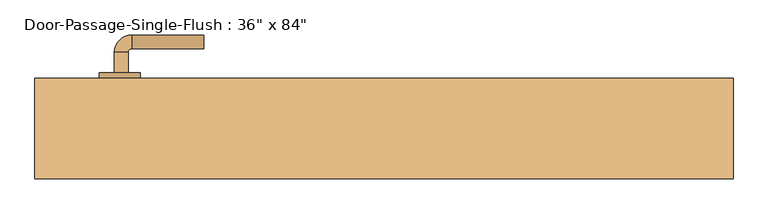
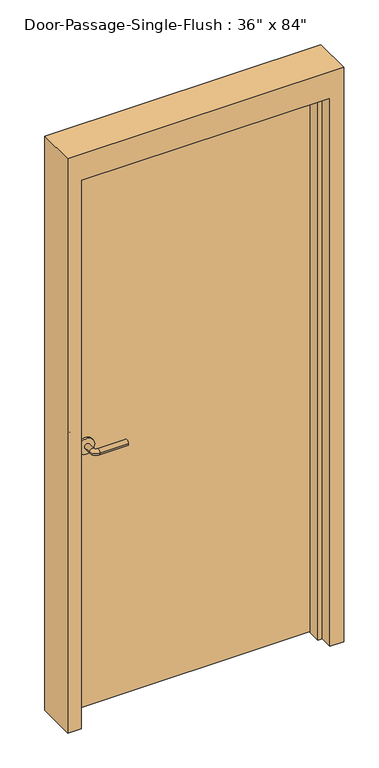
"""IFC4 building model written with IfcOpenShell, lengths in millimetres: door geometry."""

from ifc_helpers import new_model, si_unit, point, frame, frame_2d, origin, origin_with_axes, place, context, project, spatial, polyline, circle_curve, ellipse_curve, trimmed, segment, composite_curve, outline, extrude, faceted_brep, source, transform, mapped, element, save
from ifc_brep_helpers import plane_surface, cylinder_surface, revolved_surface, advanced_brep


def door_70ceb761(model_context):
    return source(origin(), model_context, "Body", "SolidModel", [
        advanced_brep(
        [(-392.190625, 4.7, 1016.0), (-372.190625, 4.7, 1016.0), (-372.190625, -25.3, 1016.0), (-392.190625, -25.3, 1016.0), (-367.190625, -30.3, 1016.0), (-367.190625, -50.3, 1016.0), (-262.190625, -50.3, 1016.0), (-262.190625, -30.3, 1016.0)],
        [
            (0, 1, circle_curve(frame((-382.190625, 4.7, 1016.0), z_axis=(0.0, 1.0, 0.0), x_axis=(1.0, 0.0, 0.0)), 10.0)),
            (1, 0, circle_curve(frame((-382.190625, 4.7, 1016.0), z_axis=(0.0, 1.0, 0.0), x_axis=(1.0, 0.0, 0.0)), 10.0)),
            (1, 2),
            (2, 3, circle_curve(frame((-382.190625, -25.3, 1016.0), z_axis=(0.0, 1.0, 0.0), x_axis=(1.0, 0.0, 0.0)), 10.0)),
            (3, 0),
            (3, 2, circle_curve(frame((-382.190625, -25.3, 1016.0), z_axis=(0.0, 1.0, 0.0), x_axis=(1.0, 0.0, 0.0)), 10.0)),
            (4, 5, circle_curve(frame((-367.190625, -40.3, 1016.0), z_axis=(-1.0, 0.0, 0.0), x_axis=(0.0, 1.0, 0.0)), 10.0)),
            (5, 3, circle_curve(frame((-367.190625, -25.3, 1016.0), z_axis=(0.0, 0.0, -1.0), x_axis=(-1.0, 0.0, 0.0)), 25.0)),
            (2, 4, circle_curve(frame((-367.190625, -25.3, 1016.0), z_axis=(0.0, 0.0, 1.0), x_axis=(-1.0, 0.0, 0.0)), 5.0)),
            (5, 4, circle_curve(frame((-367.190625, -40.3, 1016.0), z_axis=(-1.0, 0.0, 0.0), x_axis=(0.0, 1.0, 0.0)), 10.0)),
            (6, 7, circle_curve(frame((-262.190625, -40.3, 1016.0), z_axis=(1.0, 0.0, 0.0), x_axis=(0.0, 1.0, 0.0)), 10.0)),
            (7, 6, circle_curve(frame((-262.190625, -40.3, 1016.0), z_axis=(1.0, 0.0, 0.0), x_axis=(0.0, 1.0, 0.0)), 10.0)),
            (4, 7),
            (6, 5),
        ],
        [
            plane_surface(frame((-382.190625, 4.7, 1016.0), z_axis=(0.0, 1.0, 0.0), x_axis=(0.0, 0.0, 1.0))),
            cylinder_surface(frame((-382.190625, 4.7, 1016.0), z_axis=(0.0, 1.0, 0.0), x_axis=(1.0, 0.0, 0.0)), 10.0),
            revolved_surface(trimmed(ellipse_curve(frame((-382.190625, -25.3, 1016.0), z_axis=(0.0, -1.0, 0.0), x_axis=(1.0, 0.0, 0.0)), 10.0, 10.0), [point((-392.190625, -25.3, 1016.0))], [point((-372.190625, -25.3, 1016.0))], True, "CARTESIAN"), (-367.190625, -25.3, 1016.0), (0.0, 0.0, -1.0)),
            revolved_surface(trimmed(ellipse_curve(frame((-382.190625, -25.3, 1016.0), z_axis=(0.0, -1.0, 0.0), x_axis=(1.0, 0.0, 0.0)), 10.0, 10.0), [point((-372.190625, -25.3, 1016.0))], [point((-392.190625, -25.3, 1016.0))], True, "CARTESIAN"), (-367.190625, -25.3, 1016.0), (0.0, 0.0, -1.0)),
            plane_surface(frame((-262.190625, -40.3, 1016.0), z_axis=(1.0, 0.0, 0.0), x_axis=(0.0, 0.0, 1.0))),
            cylinder_surface(frame((-367.190625, -40.3, 1016.0), z_axis=(-1.0, 0.0, 0.0), x_axis=(0.0, 1.0, 0.0)), 10.0),
        ],
        [
            (0, [[1, 2]]),
            (1, [[3, 4, 5, -2]]),
            (1, [[-5, 6, -3, -1]]),
            (2, [[7, 8, -4, 9]]),
            (3, [[10, -9, -6, -8]]),
            (4, [[11, 12]]),
            (5, [[13, -11, 14, -7]]),
            (5, [[-14, -12, -13, -10]]),
        ],
    ),
        extrude(outline(composite_curve([segment(trimmed(circle_curve(frame_2d((1016.0, -384.690625)), 30.0), [point((1016.0, -414.690625))], [point((1016.0, -354.690625))], False, "CARTESIAN"), True, "CONTINUOUS"), segment(trimmed(circle_curve(frame_2d((1016.0, -384.690625)), 30.0), [point((1016.0, -354.690625))], [point((1016.0, -414.690625))], False, "CARTESIAN"), True, "CONTINUOUS")], self_intersect=False)), frame((0.0, 4.7, 0.0), z_axis=(0.0, 1.0, 0.0), x_axis=(0.0, 0.0, 1.0)), (0.0, 0.0, 1.0), 8.0),
        advanced_brep(
        [(-392.190625, 65.15, 1016.0), (-372.190625, 65.15, 1016.0), (-392.190625, 95.15, 1016.0), (-372.190625, 95.15, 1016.0), (-367.190625, 100.15, 1016.0), (-367.190625, 120.15, 1016.0), (-262.190625, 120.15, 1016.0), (-262.190625, 100.15, 1016.0)],
        [
            (0, 1, circle_curve(frame((-382.190625, 65.15, 1016.0), z_axis=(0.0, -1.0, 0.0), x_axis=(1.0, 0.0, 0.0)), 10.0)),
            (1, 0, circle_curve(frame((-382.190625, 65.15, 1016.0), z_axis=(0.0, -1.0, 0.0), x_axis=(1.0, 0.0, 0.0)), 10.0)),
            (0, 2),
            (2, 3, circle_curve(frame((-382.190625, 95.15, 1016.0), z_axis=(0.0, -1.0, 0.0), x_axis=(1.0, 0.0, 0.0)), 10.0)),
            (3, 1),
            (3, 2, circle_curve(frame((-382.190625, 95.15, 1016.0), z_axis=(0.0, -1.0, 0.0), x_axis=(1.0, 0.0, 0.0)), 10.0)),
            (4, 3, circle_curve(frame((-367.190625, 95.15, 1016.0), z_axis=(0.0, 0.0, 1.0), x_axis=(-1.0, 0.0, 0.0)), 5.0)),
            (2, 5, circle_curve(frame((-367.190625, 95.15, 1016.0), z_axis=(0.0, 0.0, -1.0), x_axis=(-1.0, 0.0, 0.0)), 25.0)),
            (5, 4, circle_curve(frame((-367.190625, 110.15, 1016.0), z_axis=(-1.0, 0.0, 0.0), x_axis=(0.0, -1.0, 0.0)), 10.0)),
            (4, 5, circle_curve(frame((-367.190625, 110.15, 1016.0), z_axis=(-1.0, 0.0, 0.0), x_axis=(0.0, -1.0, 0.0)), 10.0)),
            (6, 7, circle_curve(frame((-262.190625, 110.15, 1016.0), z_axis=(1.0, 0.0, 0.0), x_axis=(0.0, -1.0, 0.0)), 10.0)),
            (7, 6, circle_curve(frame((-262.190625, 110.15, 1016.0), z_axis=(1.0, 0.0, 0.0), x_axis=(0.0, -1.0, 0.0)), 10.0)),
            (5, 6),
            (7, 4),
        ],
        [
            plane_surface(frame((-382.190625, 65.15, 1016.0), z_axis=(0.0, -1.0, 0.0), x_axis=(0.0, 0.0, 1.0))),
            cylinder_surface(frame((-382.190625, 65.15, 1016.0), z_axis=(0.0, -1.0, 0.0), x_axis=(1.0, 0.0, 0.0)), 10.0),
            revolved_surface(trimmed(ellipse_curve(frame((-382.190625, 95.15, 1016.0), z_axis=(0.0, -1.0, 0.0), x_axis=(1.0, 0.0, 0.0)), 10.0, 10.0), [point((-392.190625, 95.15, 1016.0))], [point((-372.190625, 95.15, 1016.0))], True, "CARTESIAN"), (-367.190625, 95.15, 1016.0), (0.0, 0.0, -1.0)),
            revolved_surface(trimmed(ellipse_curve(frame((-382.190625, 95.15, 1016.0), z_axis=(0.0, -1.0, 0.0), x_axis=(1.0, 0.0, 0.0)), 10.0, 10.0), [point((-372.190625, 95.15, 1016.0))], [point((-392.190625, 95.15, 1016.0))], True, "CARTESIAN"), (-367.190625, 95.15, 1016.0), (0.0, 0.0, -1.0)),
            plane_surface(frame((-262.190625, 110.15, 1016.0), z_axis=(1.0, 0.0, 0.0), x_axis=(0.0, 0.0, 1.0))),
            cylinder_surface(frame((-367.190625, 110.15, 1016.0), z_axis=(-1.0, 0.0, 0.0), x_axis=(0.0, -1.0, 0.0)), 10.0),
        ],
        [
            (0, [[1, 2]]),
            (1, [[-1, 3, 4, 5]]),
            (1, [[-2, -5, 6, -3]]),
            (2, [[7, -4, 8, 9]]),
            (3, [[-8, -6, -7, 10]]),
            (4, [[11, 12]]),
            (5, [[-9, 13, -12, 14]]),
            (5, [[-10, -14, -11, -13]]),
        ],
    ),
        extrude(outline(composite_curve([segment(trimmed(circle_curve(frame_2d((1016.0, -384.690625)), 30.0), [point((1016.0, -414.690625))], [point((1016.0, -354.690625))], False, "CARTESIAN"), True, "CONTINUOUS"), segment(trimmed(circle_curve(frame_2d((1016.0, -384.690625)), 30.0), [point((1016.0, -354.690625))], [point((1016.0, -414.690625))], False, "CARTESIAN"), True, "CONTINUOUS")], self_intersect=False)), frame((0.0, 57.15, 0.0), z_axis=(0.0, 1.0, 0.0), x_axis=(0.0, 0.0, 1.0)), (0.0, 0.0, 1.0), 8.0),
        faceted_brep([(457.2, 7.9375, 0.0), (457.2, 57.15, 0.0), (508.0, 57.15, 0.0), (508.0, -88.9, 0.0), (457.2, -88.9, 0.0), (457.2, -39.6875, 0.0), (441.325, -39.6875, 0.0), (441.325, 7.9375, 0.0), (457.2, 7.9375, 2133.6), (457.2, 57.15, 2133.6), (-457.2, 57.15, 2133.6), (-457.2, 57.15, 0.0), (-508.0, 57.15, 0.0), (-508.0, 57.15, 2235.2), (508.0, 57.15, 2235.2), (508.0, -88.9, 2235.2), (-508.0, -88.9, 2235.2), (-508.0, -88.9, 0.0), (-457.2, -88.9, 0.0), (-457.2, -88.9, 2133.6), (457.2, -88.9, 2133.6), (457.2, -39.6875, 2133.6), (-457.2, -39.6875, 2133.6), (-457.2, -39.6875, 0.0), (-441.325, -39.6875, 0.0), (-441.325, -39.6875, 2117.725), (441.325, -39.6875, 2117.725), (441.325, 7.9375, 2117.725), (-441.325, 7.9375, 2117.725), (-441.325, 7.9375, 0.0), (-457.2, 7.9375, 0.0), (-457.2, 7.9375, 2133.6)], [[[0, 1, 2, 3, 4, 5, 6, 7]], [[1, 0, 8, 9]], [[2, 1, 9, 10, 11, 12, 13, 14]], [[3, 2, 14, 15]], [[4, 3, 15, 16, 17, 18, 19, 20]], [[5, 4, 20, 21]], [[6, 5, 21, 22, 23, 24, 25, 26]], [[7, 6, 26, 27]], [[0, 7, 27, 28, 29, 30, 31, 8]], [[9, 8, 31, 10]], [[20, 19, 22, 21]], [[26, 25, 28, 27]], [[12, 11, 30, 29, 24, 23, 18, 17]], [[11, 10, 31, 30]], [[13, 12, 17, 16]], [[19, 18, 23, 22]], [[25, 24, 29, 28]], [[15, 14, 13, 16]]]),
        extrude(outline(polyline([(457.2, 12.7), (-457.2, 12.7), (-457.2, 57.15), (457.2, 57.15), (457.2, 12.7)])), origin_with_axes(), (0.0, 0.0, 1.0), 2133.6),
    ])


if __name__ == "__main__":
    model = new_model("IFC4")
    model_context = context("Model", 3, world=origin())
    ifc_project = project(units=[si_unit("LENGTHUNIT", "METRE", prefix="MILLI")], contexts=[model_context])
    site = spatial("IfcSite", under=ifc_project)
    building = spatial("IfcBuilding", under=site)
    placement = place(None, origin())
    door_shape = door_70ceb761(model_context)
    element("IfcDoor", 1, ObjectType="Door-Passage-Single-Flush : 36\" x 84\"", at=placement, inside=building, context=model_context, shape_type="MappedRepresentation", body=[
        mapped(door_shape, transform((0.0, 0.0, 0.0), x_axis=(1.0, 0.0, 0.0), y_axis=(0.0, 1.0, 0.0), z_axis=(0.0, 0.0, 1.0))),
    ])
    save(model, "model.ifc")

# Revit data of these elements
# Type "Door-Passage-Single-Flush : 36\" x 84\""
#   Type Mark = "11"
#   Assembly Code = "B2030200"
#   Analytic Construction = "Wooden"
#   Thickness = 0' - 1 3/4"
#   Thermal Resistance (R) = 2.5876 (h·ft²·°F)/BTU
#   Swing Angle [instance default] = 90.00°
#   Strike Height = 3' - 4"
#   Rough Width [instance default] = 3' - 4"
#   Rough Height [instance default] = 7' - 4"
#   MF Opening Height [instance default] = 0' - 4"
#   MF Opening Width [instance default] = 0' - 4"
#   Inset Calculate [instance default] = 0' - 4"
#   Masonry Inset [instance default] = 0' - 1"
#   Height = 7' - 0"
#   Width = 3' - 0"
#   Heat Transfer Coefficient (U) = 0.3865 BTU/(h·ft²·°F)
#   Masonry Frame Depth = 0' - 5 3/4"
#   Masonry Frame [instance default] = yes
#   Function = 1
#   Dry Wall Frame [instance default] = no
#   Define Thermal Properties by = 1
#   Panel Material = Wood - Birch
#   Frame Material = Metal - Paint Finish - Grey
#   Door Handle Material = Aluminum
#   Visual Light Transmittance = 0
#   Solar Heat Gain Coefficient = 0
#   Wall Closure = (empty or 0)
# Element 1 (IfcDoor, "Door-Passage-Single-Flush : 36\" x 84\"")
#   Materials on its faces: "Aluminum", "Metal - Paint Finish - Grey", "Wood - Birch"
# Materials
#   "Wood - Birch": class "Wood", colour RGB 173 132 96, transparency 0, Cost = 0
#   "Metal - Paint Finish - Grey": class "Paint", colour RGB 178 178 178, transparency 0, Cost = 0
#   "Aluminum": class "Metal", colour RGB 244 245 246, transparency 0, Description = "Aluminum 6061", Cost = 0
